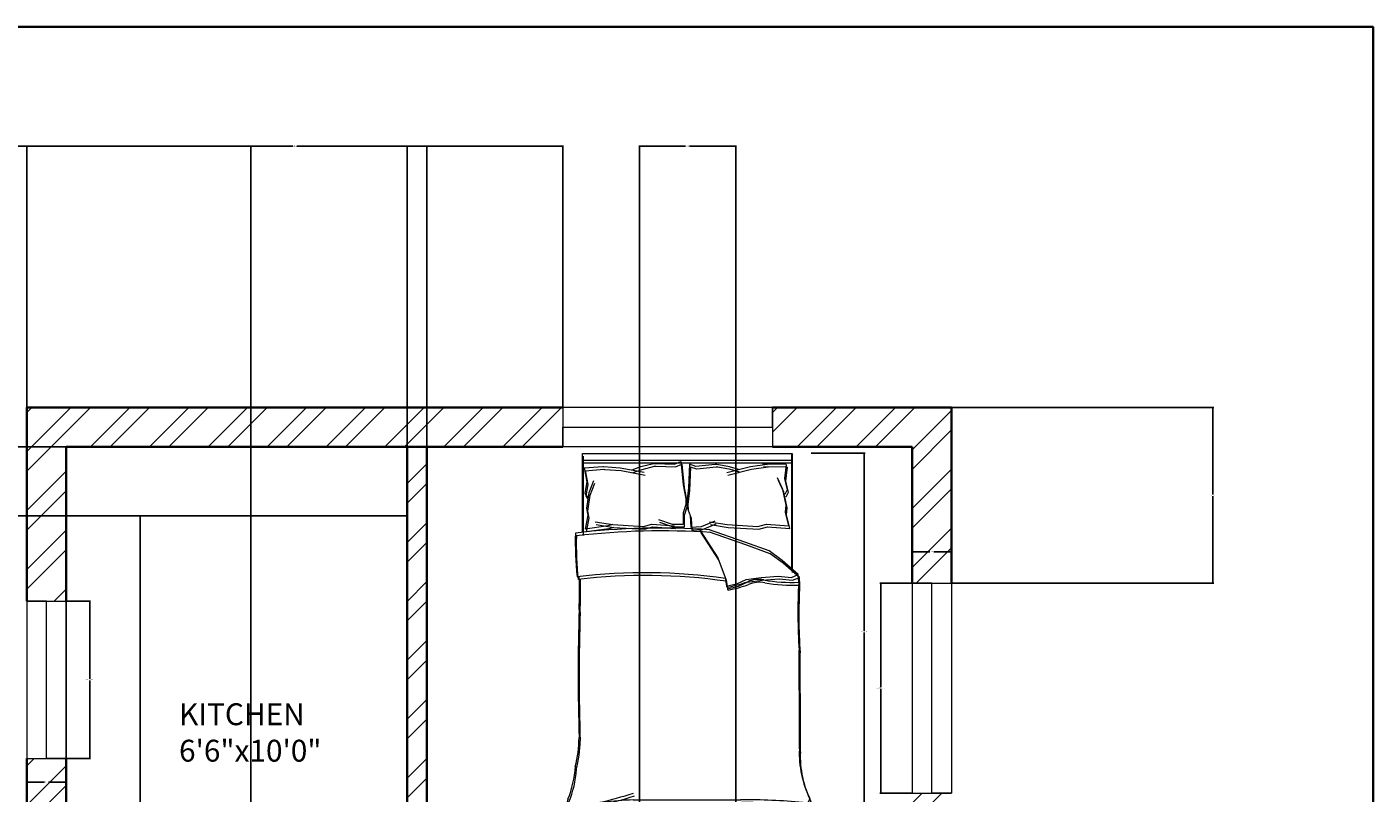
# Model space of a CAD drawing. Units: inches. Extents: x 2552 to 3217, y 1417 to 2737.
# Tile 25 of 25: x 2909 to 3217, y 2561 to 2737. Entities that reach past the tile are written whole.
import ezdxf

# ---------------------------------------------------------------- set-up
doc = ezdxf.new("R2010")
doc.units = ezdxf.units.IN
for name, color, linetype, lineweight in [('A-ANNO-DIMS', 2, 'Continuous', 18), ('A-ANNO-TTLB', 7, 'Continuous', 35), ('A-AREA-IDEN', 7, 'Continuous', 18), ('A-FLOR-CASE', 9, 'Continuous', 18), ('A-FURN', 8, 'Continuous', 13), ('A-GLAZ', 161, 'Continuous', 18), ('A-WALL', 7, 'Continuous', 35), ('A-WALL-PATT', 217, 'Continuous', 13)]:
    doc.layers.add(name, color=color, linetype=linetype, lineweight=lineweight)
doc.styles.get("Standard").update_dxf_attribs({"font": 'arial.ttf'})
doc.dimstyles.get("Standard").update_dxf_attribs({"dimtxt": 0.18, "dimasz": 0.18, "dimexe": 0.18, "dimexo": 0.0625, "dimgap": 0.09, "dimtad": 0, "dimtih": 1, "dimtoh": 1, "dimdec": 4, "dimzin": 0, "dimdsep": 46, "dimtxsty": 'Standard', "dimcen": 0.09, "dimadec": 0, "dimazin": 0, "dimtfac": 1, "dimtdec": 4, "dimtofl": 0, "dimtmove": 0, "dimatfit": 3, "dimfxl": 1, "dimtolj": 1, "dimtzin": 0, "dimarcsym": 0})

# ---------------------------------------------------------------- blocks, each defined once
blk = doc.blocks.new('BED-DOUBLE')
for p, q in [((3.47, 63.33), (3.47, 81.44)), ((3.47, 81.44), (51.49, 81.44)), ((3.48, 63.33), (3.48, 81.44)), ((3.7, 62.69), (3.7, 80.8)), ((3.7, 62.69), (3.7, 80.8)), ((51.27, 81.44), (51.27, 54.83)), ((51.27, 81.44), (51.27, 54.83)), ((51.49, 81.44), (51.49, 80.8)), ((51.49, 80.8), (51.49, 54.19)), ((51.49, 80.8), (51.49, 54.19)), ((3.47, 79.91), (51.27, 79.91)), ((3.48, 79.91), (51.27, 79.91)), ((3.7, 79.27), (51.49, 79.27)), ((3.7, 79.27), (51.49, 79.27)), ((3.89, 78.13), (4.47, 74.95)), ((3.89, 78.13), (4.47, 74.95)), ((3.9, 78.11), (8.18, 78.43)), ((3.9, 78.11), (8.18, 78.43)), ((4.12, 77.49), (4.7, 74.31)), ((4.12, 77.49), (4.7, 74.31)), ((4.13, 77.47), (8.41, 77.8)), ((4.13, 77.47), (8.41, 77.8)), ((8.18, 78.43), (8.28, 78.42)), ((8.18, 78.43), (8.28, 78.42)), ((8.28, 78.42), (12.11, 78.13)), ((8.28, 78.42), (12.11, 78.13)), ((8.41, 77.8), (8.51, 77.78)), ((8.41, 77.8), (8.51, 77.78)), ((8.51, 77.78), (12.34, 77.49)), ((8.51, 77.78), (12.34, 77.49)), ((12.11, 78.13), (17.6, 77.12)), ((12.11, 78.13), (17.6, 77.12)), ((12.34, 77.49), (17.83, 76.48)), ((12.34, 77.49), (17.83, 76.48)), ((14.85, 77.69), (16.88, 78.42)), ((14.85, 77.69), (16.88, 78.42)), ((15.08, 77.05), (17.11, 77.78)), ((15.08, 77.05), (17.11, 77.78)), ((16.88, 78.42), (19.77, 79.14)), ((16.88, 78.42), (19.77, 79.14)), ((17.11, 77.78), (20, 78.5)), ((17.11, 77.78), (20, 78.5)), ((19.77, 79.14), (20.09, 79.14)), ((19.77, 79.14), (20.09, 79.14)), ((20, 78.5), (20.32, 78.5)), ((20, 78.5), (20.32, 78.5)), ((20.09, 79.14), (24.54, 78.99)), ((20.09, 79.14), (24.54, 78.99)), ((20.32, 78.5), (24.77, 78.36)), ((20.32, 78.5), (24.77, 78.36)), ((24.54, 78.99), (25.98, 79.57)), ((24.54, 78.99), (25.98, 79.57)), ((24.77, 78.36), (26.21, 78.93)), ((24.77, 78.36), (26.21, 78.93)), ((25.98, 79.57), (26.56, 74.22)), ((25.98, 79.57), (26.56, 74.22)), ((26.21, 78.93), (26.79, 73.58)), ((26.21, 78.93), (26.79, 73.58)), ((27.98, 78.95), (27.73, 73.58)), ((27.98, 78.95), (27.73, 73.58)), ((28.21, 78.31), (27.96, 72.94)), ((28.21, 78.31), (27.96, 72.94)), ((29.46, 78.46), (27.98, 78.95)), ((29.46, 78.46), (27.98, 78.95)), ((29.68, 77.83), (28.21, 78.31)), ((29.68, 77.83), (28.21, 78.31)), ((33.88, 78.89), (29.46, 78.46)), ((33.88, 78.89), (29.46, 78.46)), ((34.11, 78.25), (29.68, 77.83)), ((34.11, 78.25), (29.68, 77.83)), ((34.2, 78.91), (33.88, 78.89)), ((34.2, 78.91), (33.88, 78.89)), ((34.43, 78.27), (34.11, 78.25)), ((34.43, 78.27), (34.11, 78.25)), ((37.14, 78.36), (34.2, 78.91)), ((37.14, 78.36), (34.2, 78.91)), ((37.36, 77.73), (34.43, 78.27)), ((37.36, 77.73), (34.43, 78.27)), ((41.91, 78.37), (36.49, 77.02)), ((41.91, 78.37), (36.5, 77.02)), ((42.14, 77.73), (36.72, 76.38)), ((42.14, 77.73), (36.72, 76.38)), ((39.2, 77.77), (37.14, 78.36)), ((39.2, 77.77), (37.14, 78.36)), ((39.43, 77.13), (37.36, 77.73)), ((39.43, 77.13), (37.36, 77.73)), ((45.71, 78.9), (41.91, 78.37)), ((45.71, 78.9), (41.91, 78.37)), ((45.94, 78.26), (42.14, 77.73)), ((45.94, 78.26), (42.14, 77.73)), ((50.11, 78.89), (44.71, 78.98)), ((44.71, 78.98), (45.71, 78.9)), ((50.11, 78.89), (44.71, 78.98)), ((44.71, 78.98), (45.71, 78.9)), ((50.34, 78.25), (44.94, 78.34)), ((44.94, 78.34), (45.94, 78.26)), ((50.34, 78.25), (44.94, 78.34)), ((44.94, 78.34), (45.94, 78.26)), ((50.11, 78.89), (49.73, 75.68)), ((50.11, 78.89), (49.73, 75.68)), ((50.34, 78.25), (49.96, 75.04)), ((50.34, 78.25), (49.96, 75.04)), ((4.47, 74.95), (4.04, 72.34)), ((4.47, 74.95), (4.04, 72.34)), ((4.7, 74.31), (4.27, 71.7)), ((4.7, 74.31), (4.27, 71.7)), ((5.05, 72.49), (6.06, 75.24)), ((5.05, 72.49), (6.06, 75.24)), ((5.28, 71.85), (6.29, 74.6)), ((5.28, 71.85), (6.29, 74.6)), ((26.56, 74.22), (27.14, 71.04)), ((26.56, 74.22), (27.14, 71.04)), ((49.31, 73.19), (48.13, 75.86)), ((49.31, 73.19), (48.13, 75.86)), ((49.54, 72.55), (48.36, 75.23)), ((49.54, 72.55), (48.36, 75.23)), ((49.73, 75.68), (50.33, 73.1)), ((49.73, 75.68), (50.33, 73.1)), ((49.96, 75.04), (50.56, 72.47)), ((49.96, 75.04), (50.56, 72.47)), ((4.04, 72.34), (4.62, 71.33)), ((4.04, 72.34), (4.62, 71.33)), ((4.27, 71.7), (4.85, 70.69)), ((4.27, 71.7), (4.85, 70.69)), ((4.47, 68.87), (5.05, 72.49)), ((4.47, 68.87), (5.05, 72.49)), ((4.7, 68.23), (5.28, 71.85)), ((4.7, 68.23), (5.28, 71.85)), ((26.79, 73.58), (27.37, 70.4)), ((26.79, 73.58), (27.37, 70.4)), ((27.14, 71.04), (27.14, 69.74)), ((27.14, 71.04), (27.14, 69.74)), ((27.73, 73.58), (27.35, 70.37)), ((27.73, 73.58), (27.35, 70.37)), ((27.96, 72.94), (27.58, 69.73)), ((27.96, 72.94), (27.58, 69.73)), ((50.11, 69.61), (49.31, 73.19)), ((50.11, 69.61), (49.31, 73.19)), ((50.34, 68.98), (49.54, 72.55)), ((50.34, 68.98), (49.54, 72.55)), ((50.33, 73.1), (49.81, 72.06)), ((50.33, 73.1), (49.81, 72.06)), ((50.56, 72.47), (50.04, 71.42)), ((50.56, 72.47), (50.04, 71.42)), ((4.76, 67.28), (4.47, 68.87)), ((4.76, 67.28), (4.47, 68.87)), ((4.99, 66.64), (4.7, 68.23)), ((4.99, 66.64), (4.7, 68.23)), ((27.14, 69.74), (26.56, 67.86)), ((27.14, 69.74), (26.56, 67.86)), ((26.56, 67.86), (26.56, 65.18)), ((26.56, 67.86), (26.56, 65.18)), ((27.37, 69.1), (26.79, 67.22)), ((27.37, 69.1), (26.79, 67.22)), ((27.35, 70.37), (27.44, 69.07)), ((27.35, 70.37), (27.44, 69.07)), ((27.37, 70.4), (27.37, 69.1)), ((27.37, 70.4), (27.37, 69.1)), ((27.44, 69.07), (28.13, 67.23)), ((27.44, 69.07), (28.13, 67.23)), ((27.58, 69.73), (27.66, 68.43)), ((27.58, 69.73), (27.66, 68.43)), ((27.66, 68.43), (28.36, 66.59)), ((27.66, 68.43), (28.36, 66.59)), ((49.92, 68.01), (50.11, 69.61)), ((49.92, 68.01), (50.11, 69.61)), ((50.7, 64.87), (49.92, 68.01)), ((50.7, 64.87), (49.92, 68.01)), ((50.15, 67.37), (50.34, 68.98)), ((50.15, 67.37), (50.34, 68.98)), ((4.18, 64.1), (4.76, 67.28)), ((4.18, 64.1), (4.76, 67.28)), ((9.28, 64.83), (4.18, 64.1)), ((9.28, 64.83), (4.18, 64.1)), ((4.41, 63.46), (4.99, 66.64)), ((4.41, 63.46), (4.99, 66.64)), ((6.38, 65.81), (10.41, 65.15)), ((6.38, 65.81), (10.41, 65.15)), ((6.61, 65.18), (10.64, 64.51)), ((6.61, 65.18), (10.64, 64.51)), ((10.41, 65.15), (9.28, 64.83)), ((10.41, 65.15), (9.28, 64.83)), ((10.41, 65.15), (17.42, 64.72)), ((10.41, 65.15), (17.42, 64.72)), ((17.42, 64.72), (19.38, 65.27)), ((17.42, 64.72), (19.38, 65.27)), ((19.38, 65.27), (24.52, 64.87)), ((19.38, 65.27), (24.52, 64.87)), ((24.1, 65.18), (20.96, 66.27)), ((24.1, 65.18), (20.96, 66.27)), ((24.33, 64.54), (21.19, 65.63)), ((24.33, 64.54), (21.19, 65.63)), ((26.56, 65.18), (24.1, 65.18)), ((26.56, 65.18), (24.1, 65.18)), ((26.79, 67.22), (26.79, 64.54)), ((26.79, 67.22), (26.79, 64.54)), ((28.13, 67.23), (28.3, 64.55)), ((28.13, 67.23), (28.3, 64.55)), ((28.3, 64.55), (30.75, 64.7)), ((28.3, 64.55), (30.75, 64.7)), ((28.36, 66.59), (28.53, 63.91)), ((28.36, 66.59), (28.53, 63.91)), ((30.75, 64.7), (33.82, 65.99)), ((30.75, 64.7), (33.82, 65.99)), ((30.98, 64.06), (34.05, 65.35)), ((30.98, 64.06), (34.05, 65.35)), ((32.56, 65.81), (36.6, 65.15)), ((32.56, 65.81), (36.6, 65.15)), ((32.79, 65.18), (36.82, 64.51)), ((32.79, 65.18), (36.82, 64.51)), ((36.6, 65.15), (43.61, 64.72)), ((36.6, 65.15), (43.61, 64.72)), ((43.61, 64.72), (45.57, 65.27)), ((43.61, 64.72), (45.57, 65.27)), ((45.57, 65.27), (50.7, 64.87)), ((45.57, 65.27), (50.7, 64.87)), ((50.93, 64.23), (50.15, 67.37)), ((50.93, 64.23), (50.15, 67.37)), ((9.51, 64.19), (4.41, 63.46)), ((9.51, 64.19), (4.41, 63.46)), ((10.64, 64.51), (9.51, 64.19)), ((10.64, 64.51), (9.51, 64.19)), ((10.64, 64.51), (17.65, 64.08)), ((10.64, 64.51), (17.65, 64.08)), ((17.65, 64.08), (19.61, 64.63)), ((17.65, 64.08), (19.61, 64.63)), ((19.61, 64.63), (24.74, 64.23)), ((19.61, 64.63), (24.74, 64.23)), ((26.79, 64.54), (24.33, 64.54)), ((26.79, 64.54), (24.33, 64.54)), ((28.53, 63.91), (30.98, 64.06)), ((28.53, 63.91), (30.98, 64.06)), ((30.26, 64.06), (34.45, 57.57)), ((30.26, 64.06), (34.45, 57.57)), ((30.49, 63.42), (34.68, 56.93)), ((30.49, 63.42), (34.68, 56.93)), ((40.64, 61.13), (32.31, 64.06)), ((40.64, 61.13), (32.31, 64.06)), ((40.87, 60.49), (32.53, 63.42)), ((40.87, 60.49), (32.53, 63.42)), ((36.82, 64.51), (43.83, 64.08)), ((36.82, 64.51), (43.83, 64.08)), ((43.83, 64.08), (45.79, 64.63)), ((43.83, 64.08), (45.79, 64.63)), ((45.79, 64.63), (50.93, 64.23)), ((45.79, 64.63), (50.93, 64.23)), ((46.22, 59.11), (40.64, 61.13)), ((46.22, 59.11), (40.64, 61.13)), ((46.45, 58.48), (40.87, 60.49)), ((46.45, 58.48), (40.87, 60.49)), ((49.16, 56.95), (46.22, 59.11)), ((49.16, 56.95), (46.22, 59.11)), ((34.45, 57.57), (36.15, 53.08)), ((34.45, 57.57), (36.15, 53.08)), ((34.68, 56.93), (36.38, 52.44)), ((34.68, 56.93), (36.38, 52.44)), ((49.39, 56.31), (46.45, 58.48)), ((49.39, 56.31), (46.45, 58.48)), ((52.87, 53.7), (49.16, 56.95)), ((52.87, 53.7), (49.16, 56.95)), ((53.1, 53.06), (49.39, 56.31)), ((53.1, 53.06), (49.39, 56.31)), ((36.15, 53.08), (36.46, 51.07)), ((36.15, 53.08), (36.46, 51.07)), ((36.38, 52.44), (36.69, 50.43)), ((36.38, 52.44), (36.69, 50.43)), ((38.94, 51.69), (40.95, 52.61)), ((38.94, 51.69), (40.95, 52.61)), ((40.95, 52.61), (44.36, 53.08)), ((40.95, 52.61), (44.36, 53.08)), ((41.18, 51.97), (44.59, 52.44)), ((41.18, 51.97), (44.59, 52.44)), ((44.36, 53.08), (48.23, 53.39)), ((44.36, 53.08), (48.23, 53.39)), ((44.59, 52.44), (48.46, 52.75)), ((44.59, 52.44), (48.46, 52.75)), ((48.23, 53.39), (51.33, 53.08)), ((48.23, 53.39), (51.33, 53.08)), ((48.46, 52.75), (51.56, 52.44)), ((48.46, 52.75), (51.56, 52.44)), ((51.33, 53.08), (52.87, 53.7)), ((51.33, 53.08), (52.87, 53.7)), ((51.56, 52.44), (53.1, 53.06)), ((51.56, 52.44), (53.1, 53.06)), ((52.95, 51.95), (52.87, 53.7, 3.87)), ((52.95, 51.95), (52.87, 53.7, 3.87)), ((53.18, 51.31), (53.1, 53.06, 3.87)), ((53.18, 51.31), (53.1, 53.06, 3.87)), ((36.46, 51.07), (38.94, 51.69)), ((36.46, 51.07), (38.94, 51.69)), ((36.69, 50.43), (39.17, 51.05)), ((36.69, 50.43), (39.17, 51.05)), ((39.17, 51.05), (41.18, 51.97)), ((39.17, 51.05), (41.18, 51.97)), ((15.06, 2.2), (39.68, 2.2)), ((15.06, 2.2), (39.68, 2.2)), ((15.29, 1.56), (39.91, 1.56)), ((15.29, 1.56), (39.91, 1.56))]:
    blk.add_line(p, q)
for centre, radius, start, end in [((85.16, 61.35), 83.31, 178.7218, 185.604), ((85.16, 61.35), 83.31, 178.7218, 185.604), ((21.36, -100.61), 164.97, 86.0865, 96.7821), ((21.36, -100.61), 164.97, 86.0865, 96.7821), ((85.39, 60.71), 83.31, 178.7218, 185.604), ((85.39, 60.71), 83.31, 178.7218, 185.604), ((21.59, -101.25), 164.97, 86.0865, 96.7821), ((21.59, -101.25), 164.97, 86.0865, 96.7821), ((17.76, -74.87), 129.02, 81.7845, 96.9006), ((17.76, -74.87), 129.02, 81.7845, 96.9006), ((17.98, -75.51), 129.02, 81.7845, 96.9006), ((17.98, -75.51), 129.02, 81.7845, 96.9006), ((-167.31, 50.27), 170.11, 358.4762, 1.0082), ((-167.31, 50.27), 170.11, 358.4762, 1.0082), ((-167.08, 49.63), 170.11, 358.4762, 1.0082), ((-167.08, 49.63), 170.11, 358.4762, 1.0082), ((43.74, 46.38), 6.22, 78.6608, 113.7384), ((43.74, 46.38), 6.22, 78.6608, 113.7384), ((51.33, 88.1), 36.18, 259.8763, 272.5657), ((51.33, 88.1), 36.18, 259.8763, 272.5657), ((36.64, 51), 0.185, 160.2464, 271.1377), ((36.64, 51), 0.185, 160.2464, 271.1377), ((31.15, 79.96), 29.65, 280.6617, 289.8806), ((31.15, 79.96), 29.65, 280.6617, 289.8806), ((36.86, 50.36), 0.185, 160.2464, 271.1377), ((36.86, 50.36), 0.185, 160.2464, 271.1377), ((31.38, 79.32), 29.65, 280.6617, 289.8806), ((31.38, 79.32), 29.65, 280.6617, 289.8806), ((43.97, 45.74), 6.22, 78.6608, 113.7384), ((43.97, 45.74), 6.22, 78.6608, 113.7384), ((51.56, 87.46), 36.18, 259.8763, 272.5657), ((51.56, 87.46), 36.18, 259.8763, 272.5657), ((182.27, 45.13), 129.5, 176.9791, 183.8365), ((182.27, 45.13), 129.5, 176.9791, 183.8365), ((182.49, 44.49), 129.5, 176.9791, 183.8365), ((182.49, 44.49), 129.5, 176.9791, 183.8365), ((484.82, 30.83), 482.31, 178.2277, 181.7185), ((484.82, 30.83), 482.31, 178.2277, 181.7185), ((485.05, 30.19), 482.31, 178.2277, 181.7185), ((485.05, 30.19), 482.31, 178.2277, 181.7185), ((-4508.74, 13.62), 4561.86, 0.00217, 0.28689), ((-4508.74, 13.62), 4561.86, 0.00217, 0.28689), ((-4508.51, 12.98), 4561.86, 0.00217, 0.28689), ((-4508.52, 12.98), 4561.86, 0.00217, 0.28689), ((-26.9, 16.93), 29.63, 346.0648, 358.9113), ((-26.9, 16.93), 29.63, 346.0648, 358.9113), ((-26.67, 16.29), 29.63, 346.0648, 358.9113), ((-26.67, 16.29), 29.63, 346.0648, 358.9113), ((76.16, 12.78), 23.07, 177.4714, 206.4681), ((76.16, 12.78), 23.07, 177.4714, 206.4681), ((76.39, 12.14), 23.07, 177.4714, 206.4681), ((76.39, 12.14), 23.07, 177.4714, 206.4681), ((-21.66, 11.17), 23.56, 337.9751, 356.652), ((-21.66, 11.17), 23.56, 337.9751, 356.652), ((-21.43, 10.53), 23.56, 337.9751, 356.652), ((-21.43, 10.53), 23.56, 337.9751, 356.652), ((-17.22, 105.16), 106.46, 283.3832, 287.7053), ((-17.22, 105.16), 106.46, 283.3832, 287.7053), ((-16.99, 104.52), 106.46, 283.3832, 287.7053), ((-16.99, 104.52), 106.46, 283.3832, 287.7053), ((1.09, 1.73), 1.09, 146.1736, 293.4781), ((1.09, 1.73), 1.09, 146.1736, 293.4781), ((1.32, 1.09), 1.09, 146.1736, 293.4781), ((1.32, 1.09), 1.09, 146.1736, 293.4781), ((21.43, -119.39), 121.76, 92.9958, 99.4091), ((21.43, -119.39), 121.76, 92.9958, 99.4091), ((21.66, -120.03), 121.76, 92.9958, 99.4091), ((21.65, -120.03), 121.76, 92.9958, 99.4091), ((41.15, -130.83), 133.04, 84.4998, 90.6351), ((41.15, -130.83), 133.04, 84.4998, 90.6351), ((41.38, -131.47), 133.04, 84.4998, 90.6351), ((41.38, -131.47), 133.04, 84.4998, 90.6351), ((54.41, 2.57), 1.1, 242.6588, 356.02), ((54.41, 2.57), 1.1, 242.6588, 356.02), ((54.64, 1.93), 1.1, 242.6588, 356.02), ((54.64, 1.93), 1.1, 242.6588, 356.02)]:
    blk.add_arc(centre, radius, start, end)
blk = doc.blocks.new('WIN-48')
for p, q in [((4.5, 48), (0, 48)), ((0, 48), (9, 48)), ((0, 48), (0, 0)), ((4.5, 0), (4.5, 48)), ((9, 48), (9, 0)), ((0, 0), (9, 0)), ((9, 0), (4.5, 0))]:
    blk.add_line(p, q)
blk = doc.blocks.new('WIN-36')
for p, q in [((4.5, 36), (0, 36)), ((0, 36), (9, 36)), ((0, 36), (0, 0)), ((4.5, 0), (4.5, 36)), ((9, 36), (9, 0)), ((0, 0), (9, 0)), ((9, 0), (4.5, 0))]:
    blk.add_line(p, q)
blk = doc.blocks.new('*D19')
at = {"layer": 'A-ANNO-DIMS', "color": 0, "lineweight": -2, "transparency": 16777216}
for p, q in [((3088.24, 2639.06), (3100.59, 2639.06)), ((3100.41, 2638.88), (3100.41, 2598.47)), ((3100.41, 2557.69), (3100.41, 2598.1)), ((3088.24, 2557.51), (3100.59, 2557.51))]:
    blk.add_line(p, q, dxfattribs=at)
at = {"layer": 'A-ANNO-DIMS', "color": 0, "transparency": 16777216}
for points in [[(3100.38, 2638.88), (3100.44, 2638.88), (3100.41, 2639.06)], [(3100.38, 2557.69), (3100.44, 2557.69), (3100.41, 2557.51)]]:
    blk.add_solid(points, dxfattribs=at)
at = {"layer": 'Defpoints', "color": 0, "transparency": 16777216}
for p in [(3088.18, 2639.06), (3100.41, 2639.06), (3088.18, 2557.51)]:
    blk.add_point(p, dxfattribs=at)
at = {"layer": 'A-ANNO-DIMS', "color": 0, "transparency": 16777216, "insert": (3100.41, 2598.29), "char_height": 0.18, "attachment_point": 5}
blk.add_mtext('\\A1;BED 82 TYP.', dxfattribs=at)
blk = doc.blocks.new('*D21')
at = {"layer": 'A-ANNO-DIMS', "color": 0, "lineweight": -2, "transparency": 16777216}
for p, q in [((3111.29, 2609.37), (3103.97, 2609.37)), ((3104.15, 2609.19), (3104.15, 2585.55)), ((3104.15, 2561.55), (3104.15, 2585.19)), ((3111.29, 2561.37), (3103.97, 2561.37))]:
    blk.add_line(p, q, dxfattribs=at)
at = {"layer": 'A-ANNO-DIMS', "color": 0, "transparency": 16777216}
for points in [[(3104.12, 2609.19), (3104.18, 2609.19), (3104.15, 2609.37)], [(3104.12, 2561.55), (3104.18, 2561.55), (3104.15, 2561.37)]]:
    blk.add_solid(points, dxfattribs=at)
at = {"layer": 'Defpoints', "color": 0, "transparency": 16777216}
for p in [(3104.15, 2609.37), (3111.35, 2609.37), (3111.35, 2561.37)]:
    blk.add_point(p, dxfattribs=at)
at = {"layer": 'A-ANNO-DIMS', "color": 0, "transparency": 16777216, "insert": (3104.15, 2585.37), "char_height": 0.18, "attachment_point": 5}
blk.add_mtext('\\A1;WINDOW 48 TYP.', dxfattribs=at)
blk = doc.blocks.new('*D22')
at = {"layer": 'A-ANNO-DIMS', "color": 0, "lineweight": -2, "transparency": 16777216}
for p, q in [((3111.35, 2609.43), (3111.35, 2616.75)), ((3111.53, 2616.57), (3115.4, 2616.57)), ((3120.17, 2616.57), (3116.31, 2616.57)), ((3120.35, 2609.43), (3120.35, 2616.75))]:
    blk.add_line(p, q, dxfattribs=at)
at = {"layer": 'A-ANNO-DIMS', "color": 0, "transparency": 16777216}
for points in [[(3111.53, 2616.6), (3111.53, 2616.54), (3111.35, 2616.57)], [(3120.17, 2616.6), (3120.17, 2616.54), (3120.35, 2616.57)]]:
    blk.add_solid(points, dxfattribs=at)
at = {"layer": 'Defpoints', "color": 0, "transparency": 16777216}
for p in [(3120.35, 2616.57), (3111.35, 2609.37), (3120.35, 2609.37)]:
    blk.add_point(p, dxfattribs=at)
at = {"layer": 'A-ANNO-DIMS', "color": 0, "transparency": 16777216, "insert": (3115.85, 2616.57), "char_height": 0.18, "attachment_point": 5}
blk.add_mtext('\\A1;9 TYP.', dxfattribs=at)
blk = doc.blocks.new('*D27')
at = {"layer": 'A-ANNO-DIMS', "color": 0, "lineweight": -2, "transparency": 16777216}
for p, q in [((2917.92, 2605.28), (2923.43, 2605.28)), ((2923.25, 2605.1), (2923.25, 2587.46)), ((2923.25, 2569.46), (2923.25, 2587.09)), ((2917.92, 2569.28), (2923.43, 2569.28))]:
    blk.add_line(p, q, dxfattribs=at)
at = {"layer": 'A-ANNO-DIMS', "color": 0, "transparency": 16777216}
for points in [[(2923.22, 2605.1), (2923.28, 2605.1), (2923.25, 2605.28)], [(2923.22, 2569.46), (2923.28, 2569.46), (2923.25, 2569.28)]]:
    blk.add_solid(points, dxfattribs=at)
at = {"layer": 'Defpoints', "color": 0, "transparency": 16777216}
for p in [(2917.85, 2605.28), (2923.25, 2605.28), (2917.85, 2569.28)]:
    blk.add_point(p, dxfattribs=at)
at = {"layer": 'A-ANNO-DIMS', "color": 0, "transparency": 16777216, "insert": (2923.25, 2587.28), "char_height": 0.18, "attachment_point": 5}
blk.add_mtext('\\A1;WINDOW 36 TYP.', dxfattribs=at)
blk = doc.blocks.new('*D28')
at = {"layer": 'A-ANNO-DIMS', "color": 0, "lineweight": -2, "transparency": 16777216}
for p, q in [((2908.85, 2569.21), (2908.85, 2563.7)), ((2917.85, 2569.21), (2917.85, 2563.7)), ((2909.03, 2563.88), (2912.9, 2563.88)), ((2917.67, 2563.88), (2913.81, 2563.88))]:
    blk.add_line(p, q, dxfattribs=at)
at = {"layer": 'A-ANNO-DIMS', "color": 0, "transparency": 16777216}
for points in [[(2909.03, 2563.91), (2909.03, 2563.85), (2908.85, 2563.88)], [(2917.67, 2563.91), (2917.67, 2563.85), (2917.85, 2563.88)]]:
    blk.add_solid(points, dxfattribs=at)
at = {"layer": 'Defpoints', "color": 0, "transparency": 16777216}
for p in [(2908.85, 2569.28), (2917.85, 2569.28), (2917.85, 2563.88)]:
    blk.add_point(p, dxfattribs=at)
at = {"layer": 'A-ANNO-DIMS', "color": 0, "transparency": 16777216, "insert": (2913.35, 2563.88), "char_height": 0.18, "attachment_point": 5}
blk.add_mtext('\\A1;9 TYP.', dxfattribs=at)
blk = doc.blocks.new('*D58')
at = {"layer": 'A-ANNO-DIMS', "color": 0, "lineweight": -2, "transparency": 16777216}
for p, q in [((3048.98, 2520.58), (3048.98, 2709.49)), ((3049.16, 2709.31), (3059.51, 2709.31)), ((3070.8, 2709.31), (3060.45, 2709.31)), ((3070.98, 2520.58), (3070.98, 2709.49))]:
    blk.add_line(p, q, dxfattribs=at)
at = {"layer": 'A-ANNO-DIMS', "color": 0, "transparency": 16777216}
for points in [[(3049.16, 2709.34), (3049.16, 2709.28), (3048.98, 2709.31)], [(3070.8, 2709.34), (3070.8, 2709.28), (3070.98, 2709.31)]]:
    blk.add_solid(points, dxfattribs=at)
at = {"layer": 'Defpoints', "color": 0, "transparency": 16777216}
for p in [(3070.98, 2709.31), (3048.98, 2520.51), (3070.98, 2520.51)]:
    blk.add_point(p, dxfattribs=at)
at = {"layer": 'A-ANNO-DIMS', "color": 0, "transparency": 16777216, "insert": (3059.98, 2709.31), "char_height": 0.18, "attachment_point": 5}
blk.add_mtext('\\A1;22.003', dxfattribs=at)
blk = doc.blocks.new('*D59')
at = {"layer": 'A-ANNO-DIMS', "color": 0, "lineweight": -2, "transparency": 16777216}
for p, q in [((2995.85, 2640.58), (2995.85, 2709.49)), ((2996.03, 2709.31), (2997.85, 2709.31)), ((3000.17, 2709.31), (2998.36, 2709.31)), ((3000.35, 2640.58), (3000.35, 2709.49))]:
    blk.add_line(p, q, dxfattribs=at)
at = {"layer": 'A-ANNO-DIMS', "color": 0, "transparency": 16777216}
for points in [[(2996.03, 2709.34), (2996.03, 2709.28), (2995.85, 2709.31)], [(3000.17, 2709.34), (3000.17, 2709.28), (3000.35, 2709.31)]]:
    blk.add_solid(points, dxfattribs=at)
at = {"layer": 'Defpoints', "color": 0, "transparency": 16777216}
for p in [(3000.35, 2709.31), (2995.85, 2640.51), (3000.35, 2640.51)]:
    blk.add_point(p, dxfattribs=at)
at = {"layer": 'A-ANNO-DIMS', "color": 0, "transparency": 16777216, "insert": (2998.1, 2709.31), "char_height": 0.18, "attachment_point": 5}
blk.add_mtext('\\A1;4.5', dxfattribs=at)
blk = doc.blocks.new('*D60')
at = {"layer": 'A-ANNO-DIMS', "color": 0, "lineweight": -2, "transparency": 16777216}
for p, q in [((2908.85, 2649.58), (2908.85, 2709.49)), ((2909.03, 2709.31), (2969.69, 2709.31)), ((3031.25, 2709.31), (2970.6, 2709.31)), ((3031.43, 2649.58), (3031.43, 2709.49))]:
    blk.add_line(p, q, dxfattribs=at)
at = {"layer": 'A-ANNO-DIMS', "color": 0, "transparency": 16777216}
for points in [[(2909.03, 2709.34), (2909.03, 2709.28), (2908.85, 2709.31)], [(3031.25, 2709.34), (3031.25, 2709.28), (3031.43, 2709.31)]]:
    blk.add_solid(points, dxfattribs=at)
at = {"layer": 'Defpoints', "color": 0, "transparency": 16777216}
for p in [(3031.43, 2709.31), (2908.85, 2649.51), (3031.43, 2649.51)]:
    blk.add_point(p, dxfattribs=at)
at = {"layer": 'A-ANNO-DIMS', "color": 0, "transparency": 16777216, "insert": (2970.14, 2709.31), "char_height": 0.18, "attachment_point": 5}
blk.add_mtext('\\A1;122.57', dxfattribs=at)
blk = doc.blocks.new('*D61')
at = {"layer": 'A-ANNO-DIMS', "color": 0, "lineweight": -2, "transparency": 16777216}
for p, q in [((3120.42, 2649.51), (3180.33, 2649.51)), ((3180.15, 2649.33), (3180.15, 2629.62)), ((3180.15, 2609.55), (3180.15, 2629.26)), ((3120.42, 2609.37), (3180.33, 2609.37))]:
    blk.add_line(p, q, dxfattribs=at)
at = {"layer": 'A-ANNO-DIMS', "color": 0, "transparency": 16777216}
for points in [[(3180.12, 2649.33), (3180.18, 2649.33), (3180.15, 2649.51)], [(3180.12, 2609.55), (3180.18, 2609.55), (3180.15, 2609.37)]]:
    blk.add_solid(points, dxfattribs=at)
at = {"layer": 'Defpoints', "color": 0, "transparency": 16777216}
for p in [(3120.35, 2649.51), (3180.15, 2649.51), (3120.35, 2609.37)]:
    blk.add_point(p, dxfattribs=at)
at = {"layer": 'A-ANNO-DIMS', "color": 0, "transparency": 16777216, "insert": (3180.15, 2629.44), "char_height": 0.18, "attachment_point": 5}
blk.add_mtext('\\A1;40.14', dxfattribs=at)
blk = doc.blocks.new('*D64')
at = {"layer": 'A-ANNO-DIMS', "color": 0, "lineweight": -2, "transparency": 16777216}
for p, q in [((2646.35, 1551.58), (2646.35, 2709.49)), ((2646.53, 2709.31), (2802.77, 2709.31)), ((2959.93, 2709.31), (2803.69, 2709.31)), ((2960.11, 1551.58), (2960.11, 2709.49))]:
    blk.add_line(p, q, dxfattribs=at)
at = {"layer": 'A-ANNO-DIMS', "color": 0, "transparency": 16777216}
for points in [[(2646.53, 2709.34), (2646.53, 2709.28), (2646.35, 2709.31)], [(2959.93, 2709.34), (2959.93, 2709.28), (2960.11, 2709.31)]]:
    blk.add_solid(points, dxfattribs=at)
at = {"layer": 'Defpoints', "color": 0, "transparency": 16777216}
for p in [(2960.11, 2709.31), (2646.35, 1551.51), (2960.11, 1551.51)]:
    blk.add_point(p, dxfattribs=at)
at = {"layer": 'A-ANNO-DIMS', "color": 0, "transparency": 16777216, "insert": (2803.23, 2709.31), "char_height": 0.18, "attachment_point": 5}
blk.add_mtext('\\A1;313.76', dxfattribs=at)
blk = doc.blocks.new('*D67')
at = {"layer": 'A-ANNO-DIMS', "color": 0, "lineweight": -2, "transparency": 16777216}
for p, q in [((2917.85, 2640.45), (2917.85, 1482.53)), ((2934.77, 2624.73), (2934.77, 1482.53)), ((2918.03, 1482.71), (2925.86, 1482.71)), ((2934.59, 1482.71), (2926.76, 1482.71))]:
    blk.add_line(p, q, dxfattribs=at)
at = {"layer": 'A-ANNO-DIMS', "color": 0, "transparency": 16777216}
for points in [[(2918.03, 1482.74), (2918.03, 1482.68), (2917.85, 1482.71)], [(2934.59, 1482.74), (2934.59, 1482.68), (2934.77, 1482.71)]]:
    blk.add_solid(points, dxfattribs=at)
at = {"layer": 'Defpoints', "color": 0, "transparency": 16777216}
for p in [(2917.85, 2640.51), (2934.77, 2624.79), (2934.77, 1482.71)]:
    blk.add_point(p, dxfattribs=at)
at = {"layer": 'A-ANNO-DIMS', "color": 0, "transparency": 16777216, "insert": (2926.31, 1482.71), "char_height": 0.18, "attachment_point": 5}
blk.add_mtext('\\A1;16.912', dxfattribs=at)
blk = doc.blocks.new('*D68')
at = {"layer": 'A-ANNO-DIMS', "color": 0, "lineweight": -2, "transparency": 16777216}
for p, q in [((2995.79, 2640.51), (2577.37, 2640.51)), ((2577.55, 2640.33), (2577.55, 2632.84)), ((2577.55, 2624.97), (2577.55, 2632.47)), ((2995.79, 2624.79), (2577.37, 2624.79))]:
    blk.add_line(p, q, dxfattribs=at)
at = {"layer": 'A-ANNO-DIMS', "color": 0, "transparency": 16777216}
for points in [[(2577.52, 2640.33), (2577.58, 2640.33), (2577.55, 2640.51)], [(2577.52, 2624.97), (2577.58, 2624.97), (2577.55, 2624.79)]]:
    blk.add_solid(points, dxfattribs=at)
at = {"layer": 'Defpoints', "color": 0, "transparency": 16777216}
for p in [(2995.85, 2640.51), (2577.55, 2624.79), (2995.85, 2624.79)]:
    blk.add_point(p, dxfattribs=at)
at = {"layer": 'A-ANNO-DIMS', "color": 0, "transparency": 16777216, "insert": (2577.55, 2632.65), "char_height": 0.18, "attachment_point": 5}
blk.add_mtext('\\A1;15.718', dxfattribs=at)

msp = doc.modelspace()

# ---------------------------------------------------------------- hatches: boundary and pattern name
at = {"layer": 'A-WALL-PATT'}
h = msp.add_hatch(dxfattribs=at)
h.set_pattern_fill('ANSI32', color=256)
h.paths.add_polyline_path([(2756.676, 2649.5125), (2637.3535, 2649.5125), (2637.3535, 2617.9626), (2641.8535, 2617.9626), (2646.3535, 2617.9626), (2646.3535, 2640.5125), (2724.3535, 2640.5125), (2724.3535, 2520.5125), (2720.299, 2520.5125), (2720.299, 2516.0125), (2733.4075, 2516.0125), (2733.4075, 2518.2213), (2733.4075, 2520.5125), (2728.8535, 2520.5125), (2728.8535, 2640.5125), (2756.676, 2640.5125)])
h.paths.add_polyline_path([(2848.8535, 2649.5125), (2804.676, 2649.5125), (2804.676, 2640.5125), (2839.8535, 2640.5125), (2839.8535, 2598.3517), (2848.8535, 2598.3517)])
h.paths.add_polyline_path([(2646.3535, 2516.0125), (2697.9593, 2516.0125), (2697.9593, 2518.2625), (2697.9593, 2520.5125), (2646.3535, 2520.5125), (2646.3535, 2581.9626), (2637.3535, 2581.9626), (2637.3535, 2364.3298), (2646.3535, 2364.3298), (2646.3535, 2387.0125), (2724.3535, 2387.0125), (2724.3535, 2267.0125), (2721.0443, 2267.0125), (2721.0443, 2262.5125), (2733.7854, 2262.5125), (2733.7854, 2264.7625), (2733.7854, 2267.0125), (2728.8535, 2267.0125), (2728.8535, 2387.0125), (2839.8535, 2387.0125), (2839.8535, 2363.8387), (2848.8535, 2363.8387), (2848.8535, 2403.7415), (2844.3535, 2403.7415), (2839.8535, 2403.7415), (2839.8535, 2396.0125), (2646.3535, 2396.0125)])
h.paths.add_polyline_path([(2848.8535, 2550.3517), (2844.3535, 2550.3517), (2839.8535, 2550.3517), (2839.8535, 2520.5125), (2801.9195, 2520.5125), (2801.9195, 2518.2625), (2801.9195, 2516.0125), (2839.8535, 2516.0125), (2839.8535, 2507.5813), (2848.8535, 2507.5813)], flags=17)
h.paths.add_polyline_path([(2848.8535, 2483.5813), (2844.3535, 2483.5813), (2839.8535, 2483.5813), (2839.8535, 2468.0125), (2773.8535, 2468.0125), (2773.8535, 2516.0125), (2778.1336, 2516.0125), (2778.1336, 2520.5125), (2766.696, 2520.5125), (2766.696, 2518.2625), (2766.696, 2516.0125), (2769.3535, 2516.0125), (2769.3535, 2463.5125), (2839.8535, 2463.5125), (2839.8535, 2431.0782), (2848.8535, 2431.0782)], flags=17)
h.paths.add_polyline_path([(2917.8535, 2569.2764), (2913.3535, 2569.2764), (2908.8535, 2569.2764), (2908.8535, 2433.001), (2917.8535, 2433.001), (2917.8535, 2516.0125), (2967.486, 2516.0125), (2967.486, 2520.5125), (2917.8535, 2520.5125)])
h.paths.add_polyline_path([(3000.3535, 2640.5125), (2995.8535, 2640.5125), (2995.8535, 2520.5125), (2990.688, 2520.5125), (2990.688, 2516.0125), (3004.0844, 2516.0125), (3004.0844, 2518.2625), (3004.0844, 2520.5125), (3000.3535, 2520.5125)])
h.paths.add_polyline_path([(3120.3535, 2561.3689), (3115.8535, 2561.3689), (3111.3535, 2561.3689), (3111.3535, 2520.5125), (3070.9814, 2520.5125), (3070.9814, 2518.2625), (3070.9814, 2516.0125), (3111.3535, 2516.0125), (3111.3535, 2505.1841), (3120.3535, 2505.1841)])
h.paths.add_polyline_path([(3120.3535, 2481.1841), (3115.8535, 2481.1841), (3111.3535, 2481.1841), (3111.3535, 2468.0125), (3045.3535, 2468.0125), (3045.3535, 2516.0125), (3048.9787, 2516.0125), (3048.9787, 2520.5125), (3036.3395, 2520.5125), (3036.3395, 2516.0125), (3040.8535, 2516.0125), (3040.8535, 2463.5125), (3111.3535, 2463.5125), (3111.3535, 2396.0125), (2917.8535, 2396.0125), (2917.8535, 2403.4124), (2913.3535, 2403.4124), (2908.8535, 2403.4124), (2908.8535, 2182.5756), (2917.8535, 2182.5756), (2917.8535, 2262.5125), (2968.001, 2262.5125), (2968.001, 2264.7625), (2968.001, 2267.0125), (2917.8535, 2267.0125), (2917.8535, 2387.0125), (3111.3535, 2387.0125), (3111.3535, 2352.2435), (3120.3535, 2352.2435)])
h.paths.add_polyline_path([(3120.3535, 2304.2435), (3115.8535, 2304.2435), (3111.3535, 2304.2435), (3111.3535, 2267.0125), (3073.8616, 2267.0125), (3073.8616, 2264.7625), (3073.8616, 2262.5125), (3111.3535, 2262.5125), (3111.3535, 2252.376), (3120.3535, 2252.376)], flags=17)
h.paths.add_polyline_path([(3120.3535, 2228.376), (3115.8535, 2228.376), (3111.3535, 2228.376), (3111.3535, 2214.5125), (3045.3535, 2214.5125), (3045.3535, 2262.5125), (3049.3096, 2262.5125), (3049.3096, 2267.0125), (3035.0125, 2267.0125), (3035.0125, 2262.5125), (3040.8535, 2262.5125), (3040.8535, 2210.0125), (3111.3535, 2210.0125), (3111.3535, 2142.5125), (2917.8535, 2142.5125), (2917.8535, 2150.2408), (2913.3535, 2150.2408), (2908.8535, 2150.2408), (2908.8535, 1924.9905), (2917.8535, 1924.9905), (2917.8535, 2009.0125), (2971.959, 2009.0125), (2971.959, 2011.2625), (2971.959, 2013.5125), (2917.8535, 2013.5125), (2917.8535, 2133.5125), (2995.8535, 2133.5125), (2995.8535, 2013.5125), (2992.1797, 2013.5125), (2992.1797, 2009.0125), (3004.3344, 2009.0125), (3004.3344, 2011.2625), (3004.3344, 2013.5125), (3000.3535, 2013.5125), (3000.3535, 2133.5125), (3111.3535, 2133.5125), (3111.3535, 2115.0291), (3120.3535, 2115.0291)])
h.paths.add_polyline_path([(3000.3535, 2387.0125), (2995.8535, 2387.0125), (2995.8535, 2267.0125), (2991.3326, 2267.0125), (2991.3326, 2262.5125), (3004.1044, 2262.5125), (3004.1044, 2264.7625), (3004.1044, 2267.0125), (3000.3535, 2267.0125)], flags=17)
h.paths.add_polyline_path([(3120.3535, 1973.2388), (3115.8535, 1973.2388), (3111.3535, 1973.2388), (3111.3535, 1961.0125), (3045.3535, 1961.0125), (3045.3535, 2009.0125), (3048.9101, 2009.0125), (3048.9101, 2013.5125), (3037.105, 2013.5125), (3037.105, 2011.2625), (3037.105, 2009.0125), (3040.8535, 2009.0125), (3040.8535, 1956.5125), (3111.3535, 1956.5125), (3111.3535, 1889.0125), (2917.8535, 1889.0125), (2917.8535, 1895.7215), (2913.3535, 1895.7215), (2908.8535, 1895.7215), (2908.8535, 1844.2217), (2917.8535, 1844.2217), (2917.8535, 1880.0125), (3111.3535, 1880.0125), (3111.3535, 1846.9541), (3120.3535, 1846.9541)])
h.paths.add_polyline_path([(3120.3535, 2067.0291), (3111.3535, 2067.0291), (3111.3535, 2013.5125), (3071.3001, 2013.5125), (3071.3001, 2009.0125), (3111.3535, 2009.0125), (3111.3535, 1997.2388), (3120.3535, 1997.2388)], flags=0)
h.paths.add_polyline_path([(3120.3535, 1798.9541), (3115.8535, 1798.9541), (3111.3535, 1798.9541), (3111.3535, 1760.0125), (3071.2497, 1760.0125), (3071.2497, 1757.7625), (3071.2497, 1755.5125), (3111.3535, 1755.5125), (3111.3535, 1746.162), (3120.3535, 1746.2478)])
h.paths.add_polyline_path([(3120.3535, 1722.2049), (3111.3535, 1722.2049), (3111.3535, 1707.5125), (3045.3535, 1707.5125), (3045.3535, 1755.5125), (3048.6624, 1755.5125), (3048.6624, 1760.0125), (3035.3703, 1760.0125), (3035.3703, 1755.5125), (3040.8535, 1755.5125), (3040.8535, 1703.0125), (3111.3535, 1703.0125), (3111.3535, 1635.5125), (2917.8535, 1635.5125), (2917.8535, 1643.1366), (2913.3535, 1643.1366), (2908.8535, 1643.1366), (2908.8535, 1626.5125), (3120.3535, 1626.5125)])
h.paths.add_polyline_path([(2917.8535, 1755.5125), (2973.2287, 1755.5125), (2973.2287, 1757.7625), (2973.2287, 1760.0125), (2917.8535, 1760.0125), (2917.8535, 1808.2217), (2913.3535, 1808.2217), (2908.8535, 1808.2217), (2908.8535, 1676.1665), (2917.8535, 1676.1665)])
h.paths.add_polyline_path([(3000.3535, 1880.0125), (2995.8535, 1880.0125), (2995.8535, 1760.0125), (2992.9329, 1760.0125), (2992.9329, 1755.5125), (3003.8766, 1755.5125), (3003.8766, 1757.7625), (3003.8766, 1760.0125), (3000.3535, 1760.0125)])
h.paths.add_polyline_path([(2848.8535, 1896.6971), (2844.3535, 1896.6971), (2839.8535, 1896.6971), (2839.8535, 1889.0125), (2646.3535, 1889.0125), (2646.3535, 2009.0125), (2700.5253, 2009.0125), (2700.5253, 2011.2625), (2700.5253, 2013.5125), (2646.3535, 2013.5125), (2646.3535, 2053.1812), (2641.8535, 2053.1812), (2637.3535, 2053.1812), (2637.3535, 1836.254), (2646.3535, 1836.254), (2646.3535, 1880.0125), (2724.3535, 1880.0125), (2724.3535, 1760.0125), (2721.2473, 1760.0125), (2721.2473, 1755.5125), (2731.9187, 1755.5125), (2731.9187, 1757.7625), (2731.9187, 1760.0125), (2728.8535, 1760.0125), (2728.8535, 1880.0125), (2839.8535, 1880.0125), (2839.8535, 1840.3813), (2848.8535, 1840.3813)])
h.paths.add_polyline_path([(2848.8535, 1792.3813), (2844.3535, 1792.3813), (2839.8535, 1792.3813), (2839.8535, 1760.0125), (2797.8845, 1760.0125), (2797.8845, 1755.5125), (2839.8535, 1755.5125), (2839.8535, 1743.3688), (2844.3535, 1743.3688), (2848.8535, 1743.3688)], flags=0)
h.paths.add_polyline_path([(2848.8535, 1719.3688), (2844.3535, 1719.3688), (2839.8535, 1719.3688), (2839.8535, 1707.5125), (2773.8535, 1707.5125), (2773.8535, 1755.5125), (2777.716, 1755.5125), (2777.716, 1760.0125), (2760.9247, 1760.0125), (2760.9247, 1757.9721), (2760.9247, 1755.5125), (2769.3535, 1755.5125), (2769.3535, 1703.0125), (2839.8535, 1703.0125), (2839.8535, 1673.0277), (2848.8535, 1672.9407)], flags=0)
h.paths.add_polyline_path([(2646.3535, 1755.5125), (2702.9171, 1755.5125), (2702.9171, 1757.7625), (2702.9171, 1760.0125), (2646.3535, 1760.0125), (2646.3535, 1800.254), (2641.8535, 1800.254), (2637.3535, 1800.254), (2637.3535, 1626.5125), (2848.8535, 1626.5125), (2848.8535, 1643.1187), (2844.3535, 1643.1187), (2839.8535, 1643.1187), (2839.8535, 1635.5125), (2646.3535, 1635.5125)])
h.paths.add_polyline_path([(2848.8535, 2148.8427), (2844.3535, 2148.8427), (2839.8535, 2148.8427), (2839.8535, 2142.5125), (2646.3535, 2142.5125), (2646.3535, 2262.5125), (2701.3562, 2262.5125), (2701.3562, 2264.7625), (2701.3562, 2267.0125), (2646.3535, 2267.0125), (2646.3535, 2328.3298), (2637.3535, 2328.3298), (2637.3535, 2089.1812), (2646.3535, 2089.1812), (2646.3535, 2133.5125), (2839.8535, 2133.5125), (2839.8535, 2097.5966), (2848.8535, 2097.5966)])
h.paths.add_polyline_path([(2728.8535, 2133.5125), (2724.3535, 2133.5125), (2724.3535, 2013.5125), (2719.6039, 2013.5125), (2719.6039, 2009.0125), (2732.5784, 2009.0125), (2732.5784, 2011.2625), (2732.5784, 2013.5125), (2728.8535, 2013.5125)])
h.paths.add_polyline_path([(2848.8535, 1970.0557), (2844.3535, 1970.0557), (2839.8535, 1970.0557), (2839.8535, 1961.0125), (2773.8535, 1961.0125), (2773.8535, 2009.0125), (2777.3388, 2009.0125), (2777.3388, 2013.5125), (2764.7681, 2013.5125), (2764.7681, 2009.0125), (2769.3535, 2009.0125), (2769.3535, 1956.5125), (2839.8535, 1956.5125), (2839.8535, 1924.7199), (2848.8535, 1924.7199)], flags=17)
h.paths.add_polyline_path([(2848.8535, 2049.5966), (2844.3535, 2049.5966), (2839.8535, 2049.5966), (2839.8535, 2013.5125), (2798.198, 2013.5125), (2798.198, 2011.2625), (2798.198, 2009.0125), (2839.8535, 2009.0125), (2839.8535, 1994.0557), (2848.8535, 1994.0557)], flags=17)
h.paths.add_polyline_path([(2848.8535, 2315.8387), (2839.8535, 2315.8387), (2839.8535, 2267.0125), (2799.3375, 2267.0125), (2799.3375, 2264.7625), (2799.3375, 2262.5125), (2839.8535, 2262.5125), (2839.8535, 2253.2843), (2848.8535, 2253.2843)], flags=17)
h.paths.add_polyline_path([(2848.8535, 2229.2843), (2839.8535, 2229.2843), (2839.8535, 2177.6936), (2848.8535, 2177.6936)], flags=17)
h.paths.add_polyline_path([(2839.8535, 2214.5125), (2773.8535, 2214.5125), (2773.8535, 2262.5125), (2777.6984, 2262.5125), (2777.6984, 2267.0125), (2763.8226, 2267.0125), (2763.8226, 2262.5125), (2769.3535, 2262.5125), (2769.3535, 2210.0125), (2839.8535, 2210.0125)], flags=17)
h.paths.add_polyline_path([(3050.32, 2520.2817), (3088.9114, 2520.2817), (3088.9114, 2538.939), (3050.32, 2538.939)], flags=9)
h = msp.add_hatch(dxfattribs=at)
h.set_pattern_fill('ANSI32', color=256)
h.paths.add_polyline_path([(3031.428, 2645.0125), (3031.428, 2649.5125), (2908.8535, 2649.5125), (2908.8535, 2605.2764), (2917.8535, 2605.2764), (2917.8535, 2640.5125), (3031.428, 2640.5125)])
h.paths.add_polyline_path([(3120.3535, 2649.5125), (3079.428, 2649.5125), (3079.428, 2640.5125), (3111.3535, 2640.5125), (3111.3535, 2609.3689), (3120.3535, 2609.3689)])

# ---------------------------------------------------------------- linework, layer by layer
at = {"layer": 'A-ANNO-TTLB'}
msp.add_lwpolyline([(2552.473, 2736.5692), (3216.7862, 2736.5692), (3216.7862, 1416.6914), (2552.473, 1416.6914)], close=True, dxfattribs=at)
at = {"layer": 'A-FLOR-CASE'}
for p, q in [((2934.7654, 2520.5125), (2934.7654, 2624.7942)), ((2934.7654, 2624.7942), (2995.8535, 2624.7942))]:
    msp.add_line(p, q, dxfattribs=at)
at = {"layer": 'A-GLAZ'}
msp.add_line((2908.8535, 2569.2764), (2908.8535, 2569.2764), dxfattribs=at)
at = {"layer": 'A-WALL'}
for p, q in [((2908.8535, 2649.5125), (2908.8535, 2605.2764)), ((2908.8535, 2649.5125), (3031.428, 2649.5125)), ((3079.428, 2649.5125), (3120.3535, 2649.5125)), ((3120.3535, 2649.5125), (3120.3535, 2609.3689)), ((2917.8535, 2640.5125), (2917.8535, 2605.2764)), ((2917.8535, 2640.5125), (3031.428, 2640.5125)), ((2995.8535, 2640.5125), (2995.8535, 2520.5125)), ((3000.3535, 2640.5125), (3000.3535, 2520.5125)), ((3079.428, 2640.5125), (3111.3535, 2640.5125)), ((3111.3535, 2640.5125), (3111.3535, 2609.3689)), ((2908.8535, 2569.2764), (2908.8535, 2433.001)), ((2917.8535, 2569.2764), (2917.8535, 2520.5125))]:
    msp.add_line(p, q, dxfattribs=at)

# ---------------------------------------------------------------- block references
at = {"layer": 'A-FURN'}
msp.add_blockref('BED-DOUBLE', (3032.4429, 2557.6168), dxfattribs=at)
at = {"layer": 'A-GLAZ', "rotation": 270}
msp.add_blockref('WIN-48', (3031.4284, 2649.512), dxfattribs=at)
at = {"layer": 'A-GLAZ'}
for name, p in [('WIN-48', (3111.354, 2561.3694)), ('WIN-36', (2908.854, 2569.2767))]:
    msp.add_blockref(name, p, dxfattribs=at)

# ---------------------------------------------------------------- texts
at = {"layer": 'A-AREA-IDEN', "insert": (2943.6492, 2581.8929), "char_height": 5, "attachment_point": 1}
msp.add_mtext_dynamic_manual_height_columns('KITCHEN\\P6\'6"x10\'0"', width=119.739736, gutter_width=12.5, heights=[0], dxfattribs=at)

# ---------------------------------------------------------------- dimensions: what is measured, and where the dimension line sits
at = {"layer": 'A-ANNO-DIMS'}
for base, p1, p2, override, picture, middle in [((2960.1089, 2709.3125), (2646.3535, 1551.5125), (2960.1089, 1551.5125), {"dimdec": 2, "dimlfac": 1, "dimrnd": 0, "dimzin": 0, "dimdsep": 46, "dimlunit": 2}, '*D64', (2803.2312, 2709.3125)), ((3031.428, 2709.3125), (2908.8535, 2649.5125), (3031.428, 2649.5125), {"dimdec": 2, "dimlfac": 1, "dimrnd": 0, "dimzin": 0, "dimdsep": 46, "dimlunit": 2}, '*D60', (2970.1408, 2709.3125)), ((3000.3535, 2709.3125), (2995.8535, 2640.5125), (3000.3535, 2640.5125), {"dimdec": 1, "dimlfac": 1, "dimrnd": 0, "dimzin": 0, "dimdsep": 46, "dimlunit": 2}, '*D59', (2998.1035, 2709.3125)), ((3070.9814, 2709.3125), (3048.9787, 2520.5125), (3070.9814, 2520.5125), {"dimdec": 3, "dimlfac": 1, "dimrnd": 0, "dimzin": 0, "dimdsep": 46, "dimlunit": 2}, '*D58', (3059.98, 2709.3125)), ((2934.7654, 1482.7125), (2917.8535, 2640.5125), (2934.7654, 2624.7942), {"dimdec": 3, "dimlfac": 1, "dimrnd": 0, "dimzin": 0, "dimdsep": 46, "dimlunit": 2}, '*D67', (2926.3094, 1482.7125))]:
    dim = msp.add_linear_dim(base=base, p1=p1, p2=p2, dimstyle='Standard', override=override, dxfattribs=at)
    dim.commit()
    dim.dimension.update_dxf_attribs({"geometry": picture, "text_midpoint": middle})
for base, p1, p2, override, picture, middle in [((3180.1535, 2649.5125), (3120.3535, 2609.3689), (3120.3535, 2649.5125), {"dimdec": 2, "dimlfac": 1, "dimrnd": 0, "dimzin": 0, "dimdsep": 46, "dimlunit": 2}, '*D61', (3180.1535, 2629.4407)), ((2577.5535, 2624.7942), (2995.8535, 2640.5125), (2995.8535, 2624.7942), {"dimdec": 3, "dimlfac": 1, "dimrnd": 0, "dimzin": 0, "dimdsep": 46, "dimlunit": 2}, '*D68', (2577.5535, 2632.6534))]:
    dim = msp.add_linear_dim(base=base, p1=p1, p2=p2, angle=90, dimstyle='Standard', override=override, dxfattribs=at)
    dim.commit()
    dim.dimension.update_dxf_attribs({"geometry": picture, "text_midpoint": middle})
for base, p1, p2, text, picture, middle in [((3100.4133, 2639.0601), (3088.181, 2557.5115), (3088.181, 2639.0601), 'BED <> TYP.', '*D19', (3100.4133, 2598.2858)), ((3104.1535, 2609.3689), (3111.3535, 2561.3689), (3111.3535, 2609.3689), 'WINDOW <> TYP.', '*D21', (3104.1535, 2585.3689)), ((2923.2535, 2605.2764), (2917.8535, 2569.2764), (2917.8535, 2605.2764), 'WINDOW <> TYP.', '*D27', (2923.2535, 2587.2764))]:
    dim = msp.add_linear_dim(base=base, p1=p1, p2=p2, angle=90, text=text, dimstyle='Standard', override={"dimdec": 0, "dimlfac": 1, "dimrnd": 0, "dimzin": 0, "dimdsep": 46, "dimlunit": 2}, dxfattribs=at)
    dim.commit()
    dim.dimension.update_dxf_attribs({"geometry": picture, "text_midpoint": middle})
for base, p1, p2, picture, middle in [((3120.3535, 2616.5689), (3111.3535, 2609.3689), (3120.3535, 2609.3689), '*D22', (3115.8535, 2616.5689)), ((2917.8535, 2563.8764), (2908.8535, 2569.2764), (2917.8535, 2569.2764), '*D28', (2913.3535, 2563.8764))]:
    dim = msp.add_linear_dim(base=base, p1=p1, p2=p2, text='<> TYP.', dimstyle='Standard', override={"dimdec": 0, "dimlfac": 1, "dimrnd": 0, "dimzin": 0, "dimdsep": 46, "dimlunit": 2}, dxfattribs=at)
    dim.commit()
    dim.dimension.update_dxf_attribs({"geometry": picture, "text_midpoint": middle})

doc.saveas('drawing.dxf')
